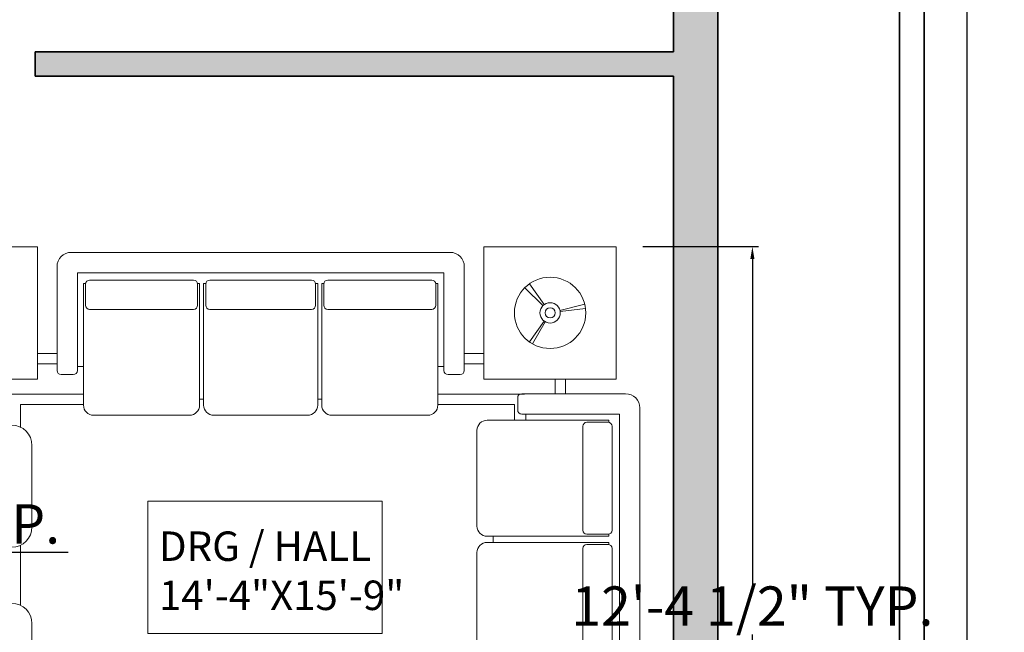
# Model space of a CAD drawing. Units: inches. Extents: x 1070 to 2371, y 645 to 1546.
# Tile 5 of 10: x 1458 to 1658, y 890 to 1014. Entities that reach past the tile are written whole.
import ezdxf

# ---------------------------------------------------------------- set-up
doc = ezdxf.new("R2010")
doc.units = ezdxf.units.IN
for name, color, linetype, lineweight in [('A-ANNO-DIMS', 2, 'Continuous', 18), ('A-AREA-IDEN', 7, 'Continuous', 18), ('A-FURN', 8, 'Continuous', 18), ('A-WALL', 7, 'Continuous', 35), ('C-PROP', 7, 'Continuous', 35)]:
    doc.layers.add(name, color=color, linetype=linetype, lineweight=lineweight)
doc.layers.add('A-WALL-PATT', color=162, linetype='Continuous', lineweight=13, true_color=0x044ac3)
doc.styles.get("Standard").update_dxf_attribs({"font": 'arial.ttf'})
doc.dimstyles.new('ISO-25', dxfattribs={"dimtxt": 8, "dimasz": 2.5, "dimexe": 1.25, "dimexo": 0.625, "dimtad": 1, "dimtih": 1, "dimtoh": 1, "dimdec": 1, "dimlunit": 3, "dimtxsty": 'Standard', "dimcen": 2.5, "dimadec": 0, "dimazin": 0, "dimtfac": 1, "dimtdec": 1, "dimtmove": 0, "dimatfit": 3, "dimfxl": 1, "dimarcsym": 0})

# ---------------------------------------------------------------- blocks, each defined once
blk = doc.blocks.new('A$C71DE5BFE')
for p, q in [((2753, 3552), (893, 3552)), ((823, 3482), (823, 2972)), ((2823, 2972), (2823, 3482)), ((923, 3452), (2723, 3452)), ((923, 2972), (923, 3452)), ((2723, 3452), (2723, 2972)), ((430.7, 3295.7), (503.4, 3397.4)), ((963.5, 3399.9), (953, 3399.9)), ((953, 3399.9), (953, 2802)), ((963, 3292), (963, 3395.7)), ((1493, 3415.7), (983, 3415.7)), ((1523, 3399.9), (1512.6, 3399.9)), ((1513, 3292), (1513, 3395.7)), ((1523, 2802), (1523, 3399.9)), ((1553.5, 3399.9), (1543, 3399.9)), ((1543, 2802), (1543, 3399.9)), ((1553, 3292), (1553, 3395.7)), ((2073, 3415.7), (1573, 3415.7)), ((2103, 3399.9), (2092.6, 3399.9)), ((2093, 3292), (2093, 3395.7)), ((2103, 2802), (2103, 3399.9)), ((2133.5, 3399.9), (2123, 3399.9)), ((2123, 2802), (2123, 3399.9)), ((2133, 3292), (2133, 3395.7)), ((2663, 3415.7), (2153, 3415.7)), ((2693, 3399.9), (2683, 3399.9)), ((2683, 3292), (2683, 3395.7)), ((2693, 2802), (2693, 3399.9)), ((3215.3, 3295.7), (3142.7, 3397.4)), ((437, 3290.4), (525.4, 3378.7)), ((3209, 3290.4), (3120.6, 3378.7)), ((353.2, 3267.1), (231.9, 3297.4)), ((3292.9, 3267.1), (3414.1, 3297.4)), ((352, 3261.2), (228, 3276.7)), ((1493, 3272), (983, 3272)), ((2073, 3272), (1573, 3272)), ((2663, 3272), (2153, 3272)), ((3294, 3261.2), (3418, 3276.7)), ((426.5, 3211.6), (488.5, 3103.1)), ((430.7, 3214.3), (503.4, 3112.6)), ((3215.3, 3214.3), (3142.7, 3112.6)), ((3219.6, 3211.6), (3157.6, 3103.1)), ((726.7, 3055), (823, 3055)), ((2823, 3055), (2919.4, 3055)), ((726.7, 3005), (823, 3005)), ((2823, 3005), (2919.4, 3005)), ((843, 2952), (903, 2952)), ((953, 2992), (923, 2992)), ((2723, 2992), (2693, 2992)), ((2743, 2952), (2803, 2952)), ((394.4, 2753.9), (394.4, 2930)), ((444.4, 2753.9), (444.4, 2930)), ((3269.4, 2930), (3269.4, 2857.9)), ((3319.4, 2930), (3319.4, 2857.9)), ((2693, 2855), (3119.4, 2855)), ((3615.1, 2857.9), (3105.1, 2857.9)), ((1543, 2832), (1523, 2832)), ((2123, 2832), (2103, 2832)), ((2693, 2805), (3069.4, 2805)), ((3069.4, 2805), (3069.4, 2727.9)), ((3085.1, 2837.9), (3085.1, 2777.9)), ((3105.1, 2757.9), (3585.1, 2757.9)), ((3125.1, 2727.9), (3125.1, 2757.9)), ((3585.1, 2757.9), (3585.1, 1527.9)), ((3685.1, 1497.9), (3685.1, 2787.9)), ((350, 2753.9), (510, 2753.9)), ((540, 2723.9), (540, 2703.9)), ((1473, 2752), (1003, 2752)), ((2053, 2752), (1593, 2752)), ((2643, 2752), (2173, 2752)), ((3532.9, 2727.9), (2935.1, 2727.9)), ((3425.1, 2717.9), (3528.7, 2717.9)), ((3532.9, 2717.5), (3532.9, 2727.9)), ((202.1, 2655.3), (206.4, 2659.6)), ((206.4, 2659.6), (210.7, 2661.9)), ((210.7, 2661.9), (213.1, 2666.2)), ((213.1, 2666.2), (217.4, 2668.5)), ((217.4, 2668.5), (219.7, 2672.9)), ((219.7, 2672.9), (224, 2672.9)), ((224, 2672.9), (228.3, 2675.2)), ((228.3, 2675.2), (232.7, 2677.2)), ((232.7, 2677.2), (245.9, 2677.2)), ((245.9, 2677.2), (250.2, 2679.5)), ((250.2, 2679.5), (254.6, 2681.5)), ((254.6, 2681.5), (256.9, 2686.1)), ((256.9, 2686.1), (261.2, 2686.1)), ((261.2, 2686.1), (265.5, 2688.1)), ((265.5, 2688.1), (270.1, 2688.1)), ((270.1, 2688.1), (274.4, 2690.5)), ((272.1, 2657.6), (276.5, 2661.9)), ((274.4, 2690.5), (283.1, 2690.5)), ((276.5, 2661.9), (281.1, 2664.2)), ((281.1, 2664.2), (283.1, 2668.5)), ((283.1, 2690.5), (287.7, 2692.5)), ((283.1, 2668.5), (285.4, 2672.9)), ((285.4, 2672.9), (289.7, 2677.2)), ((287.7, 2692.5), (305, 2692.5)), ((289.7, 2677.2), (292, 2681.5)), ((292, 2659.6), (289.7, 2655.3)), ((292, 2681.5), (296.3, 2686.1)), ((296.3, 2664.2), (292, 2659.6)), ((296.3, 2686.1), (298.6, 2690.5)), ((300.7, 2668.5), (296.3, 2664.2)), ((298.6, 2690.5), (300.7, 2694.8)), ((300.7, 2694.8), (303, 2694.8)), ((305, 2675.2), (300.7, 2668.5)), ((305, 2692.5), (309.6, 2694.8)), ((309.6, 2677.2), (305, 2675.2)), ((309.6, 2694.8), (322.6, 2694.8)), ((311.6, 2681.5), (309.6, 2677.2)), ((315.9, 2683.8), (311.6, 2681.5)), ((320.5, 2686.1), (315.9, 2683.8)), ((318.2, 2697.1), (322.6, 2697.1)), ((322.6, 2690.5), (320.5, 2686.1)), ((322.6, 2694.8), (326.9, 2697.1)), ((322.6, 2697.1), (326.9, 2694.8)), ((326.9, 2694.8), (322.6, 2690.5)), ((326.9, 2697.1), (329.2, 2697.1)), ((326.9, 2694.8), (331.5, 2686.1)), ((331.5, 2686.1), (333.5, 2681.5)), ((333.5, 2681.5), (333.5, 2677.2)), ((333.5, 2677.2), (335.8, 2672.9)), ((335.8, 2659.6), (333.5, 2655.3)), ((335.8, 2672.9), (335.8, 2659.6)), ((350, 2703.9), (600, 2703.9)), ((2885.1, 2207.9), (2885.1, 2677.9)), ((3405.1, 2187.9), (3405.1, 2697.9)), ((3548.7, 2187.9), (3548.7, 2697.9)), ((138.4, 2609.4), (143, 2611.4)), ((143, 2615.7), (147.3, 2618)), ((143, 2611.4), (143, 2615.7)), ((147.3, 2618), (149.4, 2622.4)), ((149.4, 2622.4), (154, 2624.7)), ((154, 2624.7), (158.3, 2626.7)), ((158.3, 2626.7), (162.6, 2631.3)), ((162.6, 2631.3), (166.9, 2635.6)), ((166.9, 2635.6), (171.3, 2637.7)), ((171.3, 2637.7), (175.9, 2640)), ((175.9, 2640), (180.2, 2642.3)), ((180.2, 2642.3), (184.5, 2646.6)), ((184.5, 2646.6), (188.8, 2648.6)), ((188.8, 2648.6), (193.5, 2650.9)), ((193.5, 2650.9), (197.8, 2653.2)), ((197.8, 2653.2), (202.1, 2655.3)), ((239.3, 2611.4), (241.6, 2615.7)), ((239.3, 2607.1), (239.3, 2611.4)), ((241.6, 2615.7), (243.6, 2620.4)), ((243.6, 2620.4), (248.2, 2624.7)), ((248.2, 2624.7), (250.2, 2629)), ((250.2, 2629), (252.5, 2633.3)), ((252.5, 2633.3), (256.9, 2637.7)), ((256.9, 2637.7), (259.2, 2642.3)), ((259.2, 2642.3), (261.2, 2646.6)), ((261.2, 2646.6), (263.5, 2650.9)), ((263.5, 2650.9), (267.8, 2655.3)), ((267.8, 2655.3), (272.1, 2657.6)), ((272.1, 2615.7), (267.8, 2605.1)), ((276.5, 2620.4), (272.1, 2615.7)), ((281.1, 2629), (276.5, 2624.7)), ((276.5, 2624.7), (276.5, 2620.4)), ((283.1, 2633.3), (281.1, 2629)), ((285.4, 2637.7), (283.1, 2633.3)), ((287.7, 2648.6), (285.4, 2644.3)), ((285.4, 2644.3), (285.4, 2637.7)), ((289.7, 2655.3), (287.7, 2648.6)), ((318.2, 2611.4), (315.9, 2607.1)), ((320.5, 2620.4), (318.2, 2615.7)), ((318.2, 2615.7), (318.2, 2611.4)), ((322.6, 2629), (320.5, 2624.7)), ((320.5, 2624.7), (320.5, 2620.4)), ((324.9, 2633.3), (322.6, 2629)), ((329.2, 2637.7), (324.9, 2633.3)), ((331.5, 2646.6), (329.2, 2642.3)), ((329.2, 2642.3), (329.2, 2637.7)), ((333.5, 2650.9), (331.5, 2646.6)), ((333.5, 2655.3), (333.5, 2650.9)), ((99.2, 2561.2), (103.5, 2563.2)), ((103.5, 2563.2), (105.6, 2567.6)), ((105.6, 2567.6), (110.2, 2567.6)), ((110.2, 2572.2), (114.5, 2574.2)), ((110.2, 2567.6), (110.2, 2572.2)), ((114.5, 2574.2), (116.5, 2578.5)), ((116.5, 2578.5), (118.8, 2583.1)), ((118.8, 2583.1), (123.1, 2585.2)), ((123.1, 2589.5), (127.5, 2591.8)), ((123.1, 2585.2), (123.1, 2589.5)), ((127.5, 2591.8), (129.8, 2596.1)), ((129.8, 2596.1), (134.1, 2600.5)), ((134.1, 2600.5), (136.4, 2605.1)), ((136.4, 2605.1), (138.4, 2609.4)), ((226.3, 2561.2), (228.3, 2565.5)), ((228.3, 2565.5), (230.6, 2569.9)), ((230.6, 2574.2), (232.7, 2580.8)), ((230.6, 2569.9), (230.6, 2574.2)), ((232.7, 2589.5), (235, 2594.1)), ((232.7, 2580.8), (232.7, 2589.5)), ((235, 2598.4), (237.3, 2602.8)), ((235, 2594.1), (235, 2598.4)), ((237.3, 2602.8), (239.3, 2607.1)), ((243.6, 2567.6), (241.6, 2561.2)), ((248.2, 2574.2), (243.6, 2567.6)), ((250.2, 2578.5), (248.2, 2574.2)), ((254.6, 2585.2), (250.2, 2578.5)), ((259.2, 2594.1), (254.6, 2585.2)), ((267.8, 2605.1), (259.2, 2594.1)), ((298.6, 2569.9), (294, 2561.2)), ((300.7, 2578.5), (298.6, 2569.9)), ((303, 2585.2), (300.7, 2578.5)), ((311.6, 2598.4), (303, 2589.5)), ((303, 2589.5), (303, 2585.2)), ((315.9, 2607.1), (311.6, 2598.4)), ((700, 2603.9), (700, 2203.9)), ((68.4, 2510.7), (70.7, 2515.1)), ((70.7, 2515.1), (72.7, 2519.4)), ((72.7, 2519.4), (75, 2523.7)), ((75, 2523.7), (79.3, 2528.3)), ((79.3, 2528.3), (83.7, 2530.4)), ((83.7, 2530.4), (86, 2534.7)), ((86, 2534.7), (88.3, 2539.3)), ((88.3, 2539.3), (90.3, 2543.6)), ((90.3, 2543.6), (92.6, 2547.9)), ((92.6, 2547.9), (94.6, 2552.3)), ((94.6, 2552.3), (99.2, 2556.6)), ((99.2, 2556.6), (99.2, 2561.2)), ((210.7, 2515.1), (213.1, 2519.4)), ((210.7, 2510.7), (210.7, 2515.1)), ((213.1, 2519.4), (217.4, 2526)), ((217.4, 2530.4), (219.7, 2534.7)), ((217.4, 2526), (217.4, 2530.4)), ((219.7, 2541.3), (221.7, 2547.9)), ((219.7, 2534.7), (219.7, 2541.3)), ((221.7, 2552.3), (224, 2556.6)), ((221.7, 2547.9), (221.7, 2552.3)), ((224, 2556.6), (226.3, 2561.2)), ((235, 2534.7), (232.7, 2530.4)), ((232.7, 2530.4), (232.7, 2510.7)), ((237.3, 2541.3), (235, 2534.7)), ((239.3, 2552.3), (237.3, 2545.6)), ((237.3, 2545.6), (237.3, 2541.3)), ((241.6, 2561.2), (239.3, 2556.6)), ((239.3, 2556.6), (239.3, 2552.3)), ((289.7, 2528.3), (285.4, 2519.4)), ((285.4, 2519.4), (285.4, 2499.8)), ((292, 2541.3), (289.7, 2534.7)), ((289.7, 2534.7), (289.7, 2528.3)), ((294, 2556.6), (292, 2547.9)), ((292, 2547.9), (292, 2541.3)), ((294, 2561.2), (294, 2556.6)), ((57.4, 2471.2), (59.7, 2475.5)), ((57.4, 2462.6), (57.4, 2471.2)), ((59.7, 2475.5), (61.8, 2480.2)), ((61.8, 2480.2), (64.1, 2484.5)), ((64.1, 2488.8), (66.4, 2493.1)), ((64.1, 2484.5), (64.1, 2488.8)), ((66.4, 2497.5), (68.4, 2502.1)), ((66.4, 2493.1), (66.4, 2497.5)), ((68.4, 2502.1), (68.4, 2510.7)), ((204.4, 2464.6), (206.4, 2469.2)), ((206.4, 2493.1), (208.7, 2497.5)), ((206.4, 2469.2), (206.4, 2493.1)), ((208.7, 2506.4), (210.7, 2510.7)), ((208.7, 2497.5), (208.7, 2506.4)), ((217.4, 2471.2), (215.4, 2466.9)), ((215.4, 2466.9), (215.4, 2436.3)), ((219.7, 2475.5), (217.4, 2471.2)), ((221.7, 2482.2), (219.7, 2475.5)), ((224, 2486.5), (221.7, 2482.2)), ((226.3, 2491.1), (224, 2486.5)), ((228.3, 2497.5), (226.3, 2491.1)), ((230.6, 2504.1), (228.3, 2497.5)), ((232.7, 2510.7), (230.6, 2504.1)), ((285.4, 2499.8), (276.5, 2482.2)), ((276.5, 2482.2), (276.5, 2453.6)), ((55.1, 2423), (57.4, 2427.4)), ((55.1, 2405.4), (55.1, 2423)), ((59.7, 2458.2), (57.4, 2462.6)), ((57.4, 2436.3), (59.7, 2440.6)), ((57.4, 2427.4), (57.4, 2436.3)), ((59.7, 2440.6), (59.7, 2458.2)), ((193.5, 2414.4), (197.8, 2427.4)), ((197.8, 2427.4), (199.8, 2431.7)), ((199.8, 2431.7), (202.1, 2436.3)), ((202.1, 2440.6), (204.4, 2445)), ((202.1, 2436.3), (202.1, 2440.6)), ((204.4, 2445), (204.4, 2464.6)), ((215.4, 2436.3), (206.4, 2418.7)), ((206.4, 2418.7), (206.4, 2392.5)), ((267.8, 2427.4), (259.2, 2410.1)), ((276.5, 2453.6), (267.8, 2445)), ((267.8, 2445), (267.8, 2427.4)), ((53.1, 2401.1), (55.1, 2405.4)), ((53.1, 2392.5), (53.1, 2401.1)), ((55.1, 2388.1), (53.1, 2392.5)), ((55.1, 2361.6), (55.1, 2388.1)), ((184.5, 2377.2), (186.8, 2381.5)), ((184.5, 2363.9), (184.5, 2377.2)), ((186.8, 2392.5), (188.8, 2396.8)), ((186.8, 2381.5), (186.8, 2392.5)), ((188.8, 2401.1), (191.2, 2405.4)), ((188.8, 2396.8), (188.8, 2401.1)), ((191.2, 2405.4), (193.5, 2414.4)), ((197.8, 2372.6), (195.5, 2368.2)), ((206.4, 2392.5), (197.8, 2383.5)), ((197.8, 2383.5), (197.8, 2372.6)), ((250.2, 2370.5), (248.2, 2366.2)), ((259.2, 2392.5), (250.2, 2374.9)), ((250.2, 2374.9), (250.2, 2370.5)), ((259.2, 2410.1), (259.2, 2392.5)), ((57.4, 2357.3), (55.1, 2361.6)), ((57.4, 2352.9), (57.4, 2357.3)), ((59.7, 2348.6), (57.4, 2352.9)), ((59.7, 2344.3), (59.7, 2348.6)), ((61.8, 2340), (59.7, 2344.3)), ((64.1, 2335.3), (61.8, 2340)), ((66.4, 2331), (64.1, 2335.3)), ((66.4, 2326.7), (66.4, 2331)), ((68.4, 2322.4), (66.4, 2326.7)), ((68.4, 2318), (68.4, 2322.4)), ((175.9, 2315.7), (177.9, 2322.4)), ((177.9, 2335.3), (180.2, 2342)), ((177.9, 2322.4), (177.9, 2335.3)), ((180.2, 2350.6), (182.5, 2357.3)), ((180.2, 2342), (180.2, 2350.6)), ((182.5, 2357.3), (184.5, 2363.9)), ((195.5, 2363.9), (193.5, 2359.6)), ((193.5, 2359.6), (193.5, 2274.2)), ((195.5, 2368.2), (195.5, 2363.9)), ((248.2, 2366.2), (248.2, 2307.1)), ((70.7, 2311.4), (68.4, 2318)), ((72.7, 2307.1), (70.7, 2311.4)), ((75, 2302.5), (72.7, 2307.1)), ((77.3, 2298.1), (75, 2302.5)), ((77.3, 2293.8), (77.3, 2298.1)), ((79.3, 2289.5), (77.3, 2293.8)), ((81.6, 2285.1), (79.3, 2289.5)), ((83.7, 2278.5), (81.6, 2285.1)), ((86, 2274.2), (83.7, 2278.5)), ((88.3, 2269.6), (86, 2274.2)), ((175.9, 2311.4), (175.9, 2315.7)), ((177.9, 2307.1), (175.9, 2311.4)), ((177.9, 2298.1), (177.9, 2307.1)), ((180.2, 2293.8), (177.9, 2298.1)), ((180.2, 2254.3), (180.2, 2293.8)), ((193.5, 2274.2), (195.5, 2265.2)), ((248.2, 2307.1), (245.9, 2300.4)), ((245.9, 2300.4), (245.9, 2263.2)), ((90.3, 2265.2), (88.3, 2269.6)), ((94.6, 2263.2), (90.3, 2265.2)), ((96.9, 2258.6), (94.6, 2263.2)), ((101.2, 2256.6), (96.9, 2258.6)), ((103.5, 2252.3), (101.2, 2256.6)), ((107.9, 2250), (103.5, 2252.3)), ((112.2, 2245.6), (107.9, 2250)), ((121.1, 2239), (112.2, 2245.6)), ((134.1, 2226), (121.1, 2239)), ((136.4, 2221.4), (134.1, 2226)), ((182.5, 2250), (180.2, 2254.3)), ((182.5, 2245.6), (182.5, 2250)), ((184.5, 2239), (182.5, 2245.6)), ((184.5, 2212.7), (184.5, 2239)), ((195.5, 2265.2), (195.5, 2252.3)), ((195.5, 2252.3), (197.8, 2247.9)), ((197.8, 2247.9), (197.8, 2243.3)), ((197.8, 2243.3), (199.8, 2232.4)), ((199.8, 2232.4), (199.8, 2215)), ((243.6, 2228), (241.6, 2223.7)), ((245.9, 2237), (243.6, 2232.4)), ((243.6, 2232.4), (243.6, 2228)), ((245.9, 2263.2), (248.2, 2258.6)), ((248.2, 2241.3), (245.9, 2237)), ((248.2, 2258.6), (248.2, 2241.3)), ((140.7, 2219.4), (136.4, 2221.4)), ((143, 2215), (140.7, 2219.4)), ((145, 2210.4), (143, 2215)), ((147.3, 2206.1), (145, 2210.4)), ((149.4, 2201.8), (147.3, 2206.1)), ((151.7, 2197.5), (149.4, 2201.8)), ((154, 2190.8), (151.7, 2197.5)), ((154, 2186.5), (154, 2190.8)), ((156, 2182.2), (154, 2186.5)), ((160.3, 2179.9), (156, 2182.2)), ((162.6, 2175.5), (160.3, 2179.9)), ((186.8, 2208.4), (184.5, 2212.7)), ((186.8, 2204.1), (186.8, 2208.4)), ((188.8, 2199.5), (186.8, 2204.1)), ((188.8, 2190.8), (188.8, 2199.5)), ((191.2, 2186.5), (188.8, 2190.8)), ((191.2, 2179.9), (191.2, 2186.5)), ((193.5, 2175.5), (191.2, 2179.9)), ((199.8, 2215), (202.1, 2208.4)), ((202.1, 2208.4), (202.1, 2186.5)), ((202.1, 2186.5), (204.4, 2182.2)), ((204.4, 2182.2), (204.4, 2173.2)), ((239.3, 2184.2), (237.3, 2179.9)), ((237.3, 2179.9), (237.3, 2175.5)), ((241.6, 2197.5), (239.3, 2193.1)), ((239.3, 2193.1), (239.3, 2184.2)), ((241.6, 2223.7), (241.6, 2197.5)), ((166.9, 2171.2), (162.6, 2175.5)), ((169.2, 2166.6), (166.9, 2171.2)), ((173.6, 2166.6), (169.2, 2166.6)), ((175.9, 2162.3), (173.6, 2166.6)), ((180.2, 2162.3), (175.9, 2162.3)), ((184.5, 2160.2), (180.2, 2162.3)), ((188.8, 2157.9), (184.5, 2160.2)), ((195.5, 2153.6), (188.8, 2157.9)), ((195.5, 2171.2), (193.5, 2175.5)), ((195.5, 2162.3), (195.5, 2171.2)), ((197.8, 2157.9), (195.5, 2162.3)), ((199.8, 2151.3), (195.5, 2153.6)), ((199.8, 2153.6), (197.8, 2157.9)), ((199.8, 2149.3), (199.8, 2153.6)), ((204.4, 2149.3), (199.8, 2151.3)), ((204.4, 2173.2), (206.4, 2168.9)), ((208.7, 2147), (204.4, 2149.3)), ((206.4, 2168.9), (206.4, 2164.6)), ((206.4, 2164.6), (208.7, 2160.2)), ((208.7, 2160.2), (210.7, 2155.9)), ((213.1, 2149.3), (208.7, 2147)), ((210.7, 2155.9), (213.1, 2151.3)), ((213.1, 2151.3), (213.1, 2149.3)), ((226.3, 2149.3), (213.1, 2149.3)), ((228.3, 2153.6), (226.3, 2149.3)), ((232.7, 2157.9), (228.3, 2153.6)), ((235, 2162.3), (232.7, 2157.9)), ((237.3, 2175.5), (235, 2171.2)), ((235, 2171.2), (235, 2162.3)), ((2935.1, 2157.9), (3532.9, 2157.9)), ((2935.1, 2127.9), (3532.9, 2127.9)), ((2965.1, 2137.9), (2965.1, 2157.9)), ((2965.1, 2127.9), (2965.1, 2147.9)), ((3425.1, 2167.9), (3528.7, 2167.9)), ((3532.9, 2157.9), (3532.9, 2168.4)), ((3532.9, 2117.5), (3532.9, 2127.9)), ((350, 2103.9), (600, 2103.9)), ((540, 2103.9), (540, 2083.9)), ((594.4, 1828.9), (594.4, 2103.9)), ((644.4, 1818.6), (644.4, 2114.3)), ((3405.1, 1587.9), (3405.1, 2097.9)), ((3425.1, 2117.9), (3528.7, 2117.9)), ((3548.7, 1587.9), (3548.7, 2097.9)), ((510, 2053.9), (350, 2053.9)), ((394.4, 1878.9), (394.4, 2053.9)), ((444.4, 1878.9), (444.4, 2053.9)), ((2885.1, 1607.9), (2885.1, 2077.9)), ((350, 1878.9), (510, 1878.9)), ((540, 1848.9), (540, 1828.9)), ((210.7, 1786.9), (213.1, 1791.2)), ((213.1, 1791.2), (217.4, 1793.5)), ((217.4, 1793.5), (219.7, 1797.9)), ((219.7, 1797.9), (224, 1797.9)), ((224, 1797.9), (228.3, 1800.2)), ((228.3, 1800.2), (232.7, 1802.2)), ((232.7, 1802.2), (245.9, 1802.2)), ((245.9, 1802.2), (250.2, 1804.5)), ((250.2, 1804.5), (254.6, 1806.5)), ((254.6, 1806.5), (256.9, 1811.1)), ((256.9, 1811.1), (261.2, 1811.1)), ((261.2, 1811.1), (265.5, 1813.1)), ((265.5, 1813.1), (270.1, 1813.1)), ((270.1, 1813.1), (274.4, 1815.5)), ((274.4, 1815.5), (283.1, 1815.5)), ((276.5, 1786.9), (281.1, 1789.2)), ((281.1, 1789.2), (283.1, 1793.5)), ((283.1, 1815.5), (287.7, 1817.5)), ((283.1, 1793.5), (285.4, 1797.9)), ((285.4, 1797.9), (289.7, 1802.2)), ((287.7, 1817.5), (305, 1817.5)), ((289.7, 1802.2), (292, 1806.5)), ((292, 1806.5), (296.3, 1811.1)), ((296.3, 1789.2), (292, 1784.6)), ((296.3, 1811.1), (298.6, 1815.5)), ((300.7, 1793.5), (296.3, 1789.2)), ((298.6, 1815.5), (300.7, 1819.8)), ((300.7, 1819.8), (303, 1819.8)), ((305, 1800.2), (300.7, 1793.5)), ((305, 1817.5), (309.6, 1819.8)), ((309.6, 1802.2), (305, 1800.2)), ((309.6, 1819.8), (322.6, 1819.8)), ((311.6, 1806.5), (309.6, 1802.2)), ((315.9, 1808.8), (311.6, 1806.5)), ((320.5, 1811.1), (315.9, 1808.8)), ((318.2, 1822.1), (322.6, 1822.1)), ((322.6, 1815.5), (320.5, 1811.1)), ((322.6, 1819.8), (326.9, 1822.1)), ((322.6, 1822.1), (326.9, 1819.8)), ((326.9, 1819.8), (322.6, 1815.5)), ((326.9, 1822.1), (329.2, 1822.1)), ((326.9, 1819.8), (331.5, 1811.1)), ((331.5, 1811.1), (333.5, 1806.5)), ((333.5, 1806.5), (333.5, 1802.2)), ((333.5, 1802.2), (335.8, 1797.9)), ((335.8, 1797.9), (335.8, 1784.6)), ((350, 1828.9), (600, 1828.9)), ((143, 1740.7), (147.3, 1743)), ((143, 1736.4), (143, 1740.7)), ((147.3, 1743), (149.4, 1747.4)), ((149.4, 1747.4), (154, 1749.7)), ((154, 1749.7), (158.3, 1751.7)), ((158.3, 1751.7), (162.6, 1756.3)), ((162.6, 1756.3), (166.9, 1760.6)), ((166.9, 1760.6), (171.3, 1762.7)), ((171.3, 1762.7), (175.9, 1765)), ((175.9, 1765), (180.2, 1767.3)), ((180.2, 1767.3), (184.5, 1771.6)), ((184.5, 1771.6), (188.8, 1773.6)), ((188.8, 1773.6), (193.5, 1775.9)), ((193.5, 1775.9), (197.8, 1778.2)), ((197.8, 1778.2), (202.1, 1780.3)), ((202.1, 1780.3), (206.4, 1784.6)), ((206.4, 1784.6), (210.7, 1786.9)), ((239.3, 1736.4), (241.6, 1740.7)), ((241.6, 1740.7), (243.6, 1745.4)), ((243.6, 1745.4), (248.2, 1749.7)), ((248.2, 1749.7), (250.2, 1754)), ((250.2, 1754), (252.5, 1758.3)), ((252.5, 1758.3), (256.9, 1762.7)), ((256.9, 1762.7), (259.2, 1767.3)), ((259.2, 1767.3), (261.2, 1771.6)), ((261.2, 1771.6), (263.5, 1775.9)), ((263.5, 1775.9), (267.8, 1780.3)), ((267.8, 1780.3), (272.1, 1782.6)), ((272.1, 1740.7), (267.8, 1730.1)), ((272.1, 1782.6), (276.5, 1786.9)), ((276.5, 1745.4), (272.1, 1740.7)), ((281.1, 1754), (276.5, 1749.7)), ((276.5, 1749.7), (276.5, 1745.4)), ((283.1, 1758.3), (281.1, 1754)), ((285.4, 1762.7), (283.1, 1758.3)), ((287.7, 1773.6), (285.4, 1769.3)), ((285.4, 1769.3), (285.4, 1762.7)), ((289.7, 1780.3), (287.7, 1773.6)), ((292, 1784.6), (289.7, 1780.3)), ((320.5, 1745.4), (318.2, 1740.7)), ((318.2, 1740.7), (318.2, 1736.4)), ((322.6, 1754), (320.5, 1749.7)), ((320.5, 1749.7), (320.5, 1745.4)), ((324.9, 1758.3), (322.6, 1754)), ((329.2, 1762.7), (324.9, 1758.3)), ((331.5, 1771.6), (329.2, 1767.3)), ((329.2, 1767.3), (329.2, 1762.7)), ((333.5, 1775.9), (331.5, 1771.6)), ((335.8, 1784.6), (333.5, 1780.3)), ((333.5, 1780.3), (333.5, 1775.9)), ((103.5, 1688.2), (105.6, 1692.6)), ((105.6, 1692.6), (110.2, 1692.6)), ((110.2, 1697.2), (114.5, 1699.2)), ((110.2, 1692.6), (110.2, 1697.2)), ((114.5, 1699.2), (116.5, 1703.5)), ((116.5, 1703.5), (118.8, 1708.1)), ((118.8, 1708.1), (123.1, 1710.2)), ((123.1, 1714.5), (127.5, 1716.8)), ((123.1, 1710.2), (123.1, 1714.5)), ((127.5, 1716.8), (129.8, 1721.1)), ((129.8, 1721.1), (134.1, 1725.5)), ((134.1, 1725.5), (136.4, 1730.1)), ((136.4, 1730.1), (138.4, 1734.4)), ((138.4, 1734.4), (143, 1736.4)), ((228.3, 1690.5), (230.6, 1694.9)), ((230.6, 1699.2), (232.7, 1705.8)), ((230.6, 1694.9), (230.6, 1699.2)), ((232.7, 1714.5), (235, 1719.1)), ((232.7, 1705.8), (232.7, 1714.5)), ((235, 1723.4), (237.3, 1727.8)), ((235, 1719.1), (235, 1723.4)), ((237.3, 1727.8), (239.3, 1732.1)), ((239.3, 1732.1), (239.3, 1736.4)), ((243.6, 1692.6), (241.6, 1686.2)), ((248.2, 1699.2), (243.6, 1692.6)), ((250.2, 1703.5), (248.2, 1699.2)), ((254.6, 1710.2), (250.2, 1703.5)), ((259.2, 1719.1), (254.6, 1710.2)), ((267.8, 1730.1), (259.2, 1719.1)), ((298.6, 1694.9), (294, 1686.2)), ((300.7, 1703.5), (298.6, 1694.9)), ((303, 1710.2), (300.7, 1703.5)), ((311.6, 1723.4), (303, 1714.5)), ((303, 1714.5), (303, 1710.2)), ((315.9, 1732.1), (311.6, 1723.4)), ((318.2, 1736.4), (315.9, 1732.1)), ((700, 1728.9), (700, 1328.9)), ((70.7, 1640.1), (72.7, 1644.4)), ((72.7, 1644.4), (75, 1648.7)), ((75, 1648.7), (79.3, 1653.3)), ((79.3, 1653.3), (83.7, 1655.4)), ((83.7, 1655.4), (86, 1659.7)), ((86, 1659.7), (88.3, 1664.3)), ((88.3, 1664.3), (90.3, 1668.6)), ((90.3, 1668.6), (92.6, 1672.9)), ((92.6, 1672.9), (94.6, 1677.3)), ((94.6, 1677.3), (99.2, 1681.6)), ((99.2, 1686.2), (103.5, 1688.2)), ((99.2, 1681.6), (99.2, 1686.2)), ((210.7, 1640.1), (213.1, 1644.4)), ((213.1, 1644.4), (217.4, 1651)), ((217.4, 1655.4), (219.7, 1659.7)), ((217.4, 1651), (217.4, 1655.4)), ((219.7, 1666.3), (221.7, 1672.9)), ((219.7, 1659.7), (219.7, 1666.3)), ((221.7, 1677.3), (224, 1681.6)), ((221.7, 1672.9), (221.7, 1677.3)), ((224, 1681.6), (226.3, 1686.2)), ((226.3, 1686.2), (228.3, 1690.5)), ((235, 1659.7), (232.7, 1655.4)), ((232.7, 1655.4), (232.7, 1635.7)), ((237.3, 1666.3), (235, 1659.7)), ((239.3, 1677.3), (237.3, 1670.6)), ((237.3, 1670.6), (237.3, 1666.3)), ((241.6, 1686.2), (239.3, 1681.6)), ((239.3, 1681.6), (239.3, 1677.3)), ((289.7, 1653.3), (285.4, 1644.4)), ((285.4, 1644.4), (285.4, 1624.8)), ((292, 1666.3), (289.7, 1659.7)), ((289.7, 1659.7), (289.7, 1653.3)), ((294, 1681.6), (292, 1672.9)), ((292, 1672.9), (292, 1666.3)), ((294, 1686.2), (294, 1681.6)), ((57.4, 1596.2), (59.7, 1600.5)), ((57.4, 1587.6), (57.4, 1596.2)), ((59.7, 1600.5), (61.8, 1605.2)), ((61.8, 1605.2), (64.1, 1609.5)), ((64.1, 1613.8), (66.4, 1618.1)), ((64.1, 1609.5), (64.1, 1613.8)), ((66.4, 1622.5), (68.4, 1627.1)), ((66.4, 1618.1), (66.4, 1622.5)), ((68.4, 1635.7), (70.7, 1640.1)), ((68.4, 1627.1), (68.4, 1635.7)), ((206.4, 1618.1), (208.7, 1622.5)), ((206.4, 1594.2), (206.4, 1618.1)), ((208.7, 1631.4), (210.7, 1635.7)), ((208.7, 1622.5), (208.7, 1631.4)), ((210.7, 1635.7), (210.7, 1640.1)), ((217.4, 1596.2), (215.4, 1591.9)), ((219.7, 1600.5), (217.4, 1596.2)), ((221.7, 1607.2), (219.7, 1600.5)), ((224, 1611.5), (221.7, 1607.2)), ((226.3, 1616.1), (224, 1611.5)), ((228.3, 1622.5), (226.3, 1616.1)), ((230.6, 1629.1), (228.3, 1622.5)), ((232.7, 1635.7), (230.6, 1629.1)), ((285.4, 1624.8), (276.5, 1607.2)), ((276.5, 1607.2), (276.5, 1578.6)), ((55.1, 1548), (57.4, 1552.4)), ((55.1, 1530.4), (55.1, 1548)), ((59.7, 1583.2), (57.4, 1587.6)), ((57.4, 1561.3), (59.7, 1565.6)), ((57.4, 1552.4), (57.4, 1561.3)), ((59.7, 1565.6), (59.7, 1583.2)), ((193.5, 1539.4), (197.8, 1552.4)), ((197.8, 1552.4), (199.8, 1556.7)), ((199.8, 1556.7), (202.1, 1561.3)), ((202.1, 1565.6), (204.4, 1570)), ((202.1, 1561.3), (202.1, 1565.6)), ((204.4, 1589.6), (206.4, 1594.2)), ((204.4, 1570), (204.4, 1589.6)), ((215.4, 1561.3), (206.4, 1543.7)), ((215.4, 1591.9), (215.4, 1561.3)), ((267.8, 1552.4), (259.2, 1535.1)), ((276.5, 1578.6), (267.8, 1570)), ((267.8, 1570), (267.8, 1552.4)), ((2935.1, 1557.9), (3532.9, 1557.9)), ((3125.1, 1527.9), (3125.1, 1557.9)), ((3425.1, 1567.9), (3528.7, 1567.9)), ((3532.9, 1557.9), (3532.9, 1567.9)), ((53.1, 1526.1), (55.1, 1530.4)), ((53.1, 1517.5), (53.1, 1526.1)), ((55.1, 1513.1), (53.1, 1517.5)), ((55.1, 1486.6), (55.1, 1513.1)), ((184.5, 1502.2), (186.8, 1506.5)), ((184.5, 1488.9), (184.5, 1502.2)), ((186.8, 1517.5), (188.8, 1521.8)), ((186.8, 1506.5), (186.8, 1517.5)), ((188.8, 1526.1), (191.2, 1530.4)), ((188.8, 1521.8), (188.8, 1526.1)), ((191.2, 1530.4), (193.5, 1539.4)), ((206.4, 1517.5), (197.8, 1508.5)), ((197.8, 1508.5), (197.8, 1497.6)), ((206.4, 1543.7), (206.4, 1517.5)), ((259.2, 1517.5), (250.2, 1499.9)), ((250.2, 1499.9), (250.2, 1495.5)), ((259.2, 1535.1), (259.2, 1517.5)), ((3085.1, 1507.9), (3085.1, 1447.9)), ((3585.1, 1527.9), (3105.1, 1527.9)), ((57.4, 1482.3), (55.1, 1486.6)), ((57.4, 1477.9), (57.4, 1482.3)), ((59.7, 1473.6), (57.4, 1477.9)), ((59.7, 1469.3), (59.7, 1473.6)), ((61.8, 1465), (59.7, 1469.3)), ((64.1, 1460.3), (61.8, 1465)), ((66.4, 1456), (64.1, 1460.3)), ((66.4, 1451.7), (66.4, 1456)), ((68.4, 1447.4), (66.4, 1451.7)), ((177.9, 1460.3), (180.2, 1467)), ((177.9, 1447.4), (177.9, 1460.3)), ((180.2, 1475.6), (182.5, 1482.3)), ((180.2, 1467), (180.2, 1475.6)), ((182.5, 1482.3), (184.5, 1488.9)), ((195.5, 1488.9), (193.5, 1484.6)), ((193.5, 1484.6), (193.5, 1399.2)), ((197.8, 1497.6), (195.5, 1493.2)), ((195.5, 1493.2), (195.5, 1488.9)), ((250.2, 1495.5), (248.2, 1491.2)), ((248.2, 1491.2), (248.2, 1432.1)), ((68.4, 1443), (68.4, 1447.4)), ((70.7, 1436.4), (68.4, 1443)), ((72.7, 1432.1), (70.7, 1436.4)), ((75, 1427.5), (72.7, 1432.1)), ((77.3, 1423.1), (75, 1427.5)), ((77.3, 1418.8), (77.3, 1423.1)), ((79.3, 1414.5), (77.3, 1418.8)), ((81.6, 1410.1), (79.3, 1414.5)), ((83.7, 1403.5), (81.6, 1410.1)), ((86, 1399.2), (83.7, 1403.5)), ((175.9, 1440.7), (177.9, 1447.4)), ((175.9, 1436.4), (175.9, 1440.7)), ((177.9, 1432.1), (175.9, 1436.4)), ((177.9, 1423.1), (177.9, 1432.1)), ((180.2, 1418.8), (177.9, 1423.1)), ((180.2, 1379.3), (180.2, 1418.8)), ((248.2, 1432.1), (245.9, 1425.4)), ((245.9, 1425.4), (245.9, 1388.2)), ((3105.1, 1427.9), (3615.1, 1427.9)), ((88.3, 1394.6), (86, 1399.2)), ((90.3, 1390.2), (88.3, 1394.6)), ((94.6, 1388.2), (90.3, 1390.2)), ((96.9, 1383.6), (94.6, 1388.2)), ((101.2, 1381.6), (96.9, 1383.6)), ((103.5, 1377.3), (101.2, 1381.6)), ((107.9, 1375), (103.5, 1377.3)), ((112.2, 1370.6), (107.9, 1375)), ((121.1, 1364), (112.2, 1370.6)), ((134.1, 1351), (121.1, 1364)), ((182.5, 1375), (180.2, 1379.3)), ((182.5, 1370.6), (182.5, 1375)), ((184.5, 1364), (182.5, 1370.6)), ((184.5, 1337.7), (184.5, 1364)), ((193.5, 1399.2), (195.5, 1390.2)), ((195.5, 1390.2), (195.5, 1377.3)), ((195.5, 1377.3), (197.8, 1372.9)), ((197.8, 1372.9), (197.8, 1368.3)), ((197.8, 1368.3), (199.8, 1357.4)), ((199.8, 1357.4), (199.8, 1340)), ((245.9, 1362), (243.6, 1357.4)), ((243.6, 1357.4), (243.6, 1353)), ((245.9, 1388.2), (248.2, 1383.6)), ((248.2, 1366.3), (245.9, 1362)), ((248.2, 1383.6), (248.2, 1366.3)), ((136.4, 1346.4), (134.1, 1351)), ((140.7, 1344.4), (136.4, 1346.4)), ((143, 1340), (140.7, 1344.4)), ((145, 1335.4), (143, 1340)), ((147.3, 1331.1), (145, 1335.4)), ((149.4, 1326.8), (147.3, 1331.1)), ((151.7, 1322.5), (149.4, 1326.8)), ((154, 1315.8), (151.7, 1322.5)), ((154, 1311.5), (154, 1315.8)), ((156, 1307.2), (154, 1311.5)), ((160.3, 1304.9), (156, 1307.2)), ((186.8, 1333.4), (184.5, 1337.7)), ((186.8, 1329.1), (186.8, 1333.4)), ((188.8, 1324.5), (186.8, 1329.1)), ((188.8, 1315.8), (188.8, 1324.5)), ((191.2, 1311.5), (188.8, 1315.8)), ((191.2, 1304.9), (191.2, 1311.5)), ((199.8, 1340), (202.1, 1333.4)), ((202.1, 1333.4), (202.1, 1311.5)), ((202.1, 1311.5), (204.4, 1307.2)), ((204.4, 1307.2), (204.4, 1298.2)), ((239.3, 1309.2), (237.3, 1304.9)), ((241.6, 1322.5), (239.3, 1318.1)), ((239.3, 1318.1), (239.3, 1309.2)), ((243.6, 1353), (241.6, 1348.7)), ((241.6, 1348.7), (241.6, 1322.5)), ((162.6, 1300.5), (160.3, 1304.9)), ((166.9, 1296.2), (162.6, 1300.5)), ((169.2, 1291.6), (166.9, 1296.2)), ((173.6, 1291.6), (169.2, 1291.6)), ((175.9, 1287.3), (173.6, 1291.6)), ((180.2, 1287.3), (175.9, 1287.3)), ((184.5, 1285.2), (180.2, 1287.3)), ((188.8, 1282.9), (184.5, 1285.2)), ((195.5, 1278.6), (188.8, 1282.9)), ((193.5, 1300.5), (191.2, 1304.9)), ((195.5, 1296.2), (193.5, 1300.5)), ((195.5, 1287.3), (195.5, 1296.2)), ((197.8, 1282.9), (195.5, 1287.3)), ((199.8, 1276.3), (195.5, 1278.6)), ((199.8, 1278.6), (197.8, 1282.9)), ((199.8, 1274.3), (199.8, 1278.6)), ((204.4, 1274.3), (199.8, 1276.3)), ((204.4, 1298.2), (206.4, 1293.9)), ((208.7, 1272), (204.4, 1274.3)), ((206.4, 1293.9), (206.4, 1289.6)), ((206.4, 1289.6), (208.7, 1285.2)), ((208.7, 1285.2), (210.7, 1280.9)), ((213.1, 1274.3), (208.7, 1272)), ((210.7, 1280.9), (213.1, 1276.3)), ((213.1, 1276.3), (213.1, 1274.3)), ((226.3, 1274.3), (213.1, 1274.3)), ((228.3, 1278.6), (226.3, 1274.3)), ((232.7, 1282.9), (228.3, 1278.6)), ((235, 1287.3), (232.7, 1282.9)), ((237.3, 1300.5), (235, 1296.2)), ((235, 1296.2), (235, 1287.3)), ((237.3, 1304.9), (237.3, 1300.5)), ((350, 1228.9), (600, 1228.9)), ((540, 1228.9), (540, 1208.9)), ((510, 1178.9), (350, 1178.9)), ((1322.3, 1189.3), (1792.3, 1189.3)), ((1922.3, 1189.3), (2392.3, 1189.3)), ((1272.3, 1139.3), (1272.3, 541.4)), ((1842.3, 1139.3), (1842.3, 541.4)), ((1872.3, 1139.3), (1872.3, 541.4)), ((2442.3, 541.4), (2442.3, 1139.3)), ((1842.3, 1109.3), (1862.3, 1109.3)), ((1852.3, 1109.3), (1872.3, 1109.3)), ((1142.3, 969.3), (1142.3, 459.3)), ((1222.3, 989.3), (1162.3, 989.3)), ((1242.3, 489.3), (1242.3, 969.3)), ((2472.3, 969.3), (2472.3, 489.3)), ((2552.3, 989.3), (2492.3, 989.3)), ((2572.3, 459.3), (2572.3, 969.3)), ((1242.3, 949.3), (1272.3, 949.3)), ((2442.3, 949.3), (2472.3, 949.3)), ((1282.3, 649.3), (1282.3, 545.6)), ((1302.3, 669.3), (1812.3, 669.3)), ((1832.3, 649.3), (1832.3, 545.6)), ((1882.3, 649.3), (1882.3, 545.6)), ((1902.3, 669.3), (2412.3, 669.3)), ((2432.3, 649.3), (2432.3, 545.6)), ((1272.3, 541.4), (1282.3, 541.4)), ((1831.9, 541.4), (1842.3, 541.4)), ((1872.3, 541.4), (1882.7, 541.4)), ((2431.9, 541.4), (2442.3, 541.4)), ((2472.3, 489.3), (1242.3, 489.3)), ((1302.3, 525.6), (1812.3, 525.6)), ((1902.3, 525.6), (2412.3, 525.6)), ((1212.3, 389.3), (2502.3, 389.3))]:
    blk.add_line(p, q)
for points in [[(726.7, 2930), (76.7, 2930), (76.7, 3580), (726.7, 3580)], [(2919.4, 2930), (3569.4, 2930), (3569.4, 3580), (2919.4, 3580)], [(2419.4, 1680), (2419.4, 2330), (1269.4, 2330), (1269.4, 1680)], [(2464.4, 0), (2464.4, 345), (1264.4, 345), (1264.4, 0)]]:
    blk.add_lwpolyline(points, close=True)
for points in [[(594.4, 2703.9), (594.4, 2855), (953, 2855)], [(644.4, 2693.6), (644.4, 2805), (953, 2805)], [(3069.4, 1557.9), (3069.4, 830), (2572.3, 830)], [(3269.4, 1427.9), (3269.4, 630), (2572.3, 630)], [(3319.4, 1427.9), (3319.4, 580), (2572.3, 580)], [(3119.4, 1427.9), (3119.4, 780), (2572.3, 780)], [(1142.3, 780), (594.4, 780), (594.4, 1228.9)], [(1142.3, 830), (644.4, 830), (644.4, 1239.3)], [(1142.3, 580), (394.4, 580), (394.4, 1178.9)], [(1142.3, 630), (444.4, 630), (444.4, 1178.9)]]:
    blk.add_lwpolyline(points)
for centre, radius in [((401.7, 3255), 175), ((3244.4, 3255), 175), ((401.7, 3255), 50), ((3244.4, 3255), 50), ((401.7, 3255), 25), ((3244.4, 3255), 25)]:
    blk.add_circle(centre, radius)
for centre, radius, start, end in [((893, 3482), 70, 90, 180), ((2753, 3482), 70, 0, 90), ((983, 3395.7), 20, 90, 180), ((1493, 3395.7), 20, 0, 90), ((1573, 3395.7), 20, 90, 180), ((2073, 3395.7), 20, 0, 90), ((2153, 3395.7), 20, 90, 180), ((2663, 3395.7), 20, 0, 90), ((983, 3292), 20, 180, 270), ((1493, 3292), 20, 270, 0), ((1573, 3292), 20, 180, 270), ((2073, 3292), 20, 270, 0), ((2153, 3292), 20, 180, 270), ((2663, 3292), 20, 270, 0), ((843, 2972), 20, 180, 270), ((903, 2972), 20, 270, 0), ((2743, 2972), 20, 180, 270), ((2803, 2972), 20, 270, 0), ((3105.1, 2837.9), 20, 90, 180), ((3615.1, 2787.9), 70, 0, 90), ((1003, 2802), 50, 180, 270), ((1473, 2802), 50, 270, 0), ((1593, 2802), 50, 180, 270), ((2053, 2802), 50, 270, 0), ((2173, 2802), 50, 180, 270), ((2643, 2802), 50, 270, 0), ((3105.1, 2777.9), 20, 180, 270), ((350, 2403.9), 350, 90, 270), ((510, 2723.9), 30, 0, 90), ((2935.1, 2677.9), 50, 90, 180), ((3425.1, 2697.9), 20, 90, 180), ((3528.7, 2697.9), 20, 0, 90), ((350, 2403.9), 300, 90, 270), ((600, 2603.9), 100, 0, 90), ((600, 2203.9), 100, 270, 0), ((2935.1, 2207.9), 50, 180, 270), ((3425.1, 2187.9), 20, 180, 270), ((3528.7, 2187.9), 20, 270, 0), ((2935.1, 2077.9), 50, 90, 180), ((510, 2083.9), 30, 270, 0), ((3425.1, 2097.9), 20, 90, 180), ((3528.7, 2097.9), 20, 0, 90), ((350, 1528.9), 350, 90, 270), ((510, 1848.9), 30, 0, 90), ((350, 1528.9), 300, 90, 270), ((600, 1728.9), 100, 0, 90), ((2935.1, 1607.9), 50, 180, 270), ((3425.1, 1587.9), 20, 180, 270), ((3528.7, 1587.9), 20, 270, 0), ((3105.1, 1507.9), 20, 90, 180), ((3615.1, 1497.9), 70, 270, 0), ((3105.1, 1447.9), 20, 180, 270), ((600, 1328.9), 100, 270, 0), ((510, 1208.9), 30, 270, 0), ((1322.3, 1139.3), 50, 90, 180), ((1792.3, 1139.3), 50, 0, 90), ((1922.3, 1139.3), 50, 90, 180), ((2392.3, 1139.3), 50, 0, 90), ((1162.3, 969.3), 20, 90, 180), ((1222.3, 969.3), 20, 0, 90), ((2492.3, 969.3), 20, 90, 180), ((2552.3, 969.3), 20, 0, 90), ((1302.3, 649.3), 20, 90, 180), ((1812.3, 649.3), 20, 0, 90), ((1902.3, 649.3), 20, 90, 180), ((2412.3, 649.3), 20, 0, 90), ((1302.3, 545.6), 20, 180, 270), ((1812.3, 545.6), 20, 270, 0), ((1902.3, 545.6), 20, 180, 270), ((2412.3, 545.6), 20, 270, 0), ((1212.3, 459.3), 70, 180, 270), ((2502.3, 459.3), 70, 270, 0)]:
    blk.add_arc(centre, radius, start, end)
blk = doc.blocks.new('*D12')
at = {"layer": 'A-ANNO-DIMS', "color": 0, "lineweight": -2, "transparency": 16777216}
for p, q in [((1642.74, 1408.77), (1652.12, 1408.77)), ((1650.87, 1406.27), (1650.87, 1053.48)), ((1650.87, 691.27), (1650.87, 1044.06)), ((1642.74, 688.77), (1652.12, 688.77))]:
    blk.add_line(p, q, dxfattribs=at)
at = {"layer": 'A-ANNO-DIMS', "color": 0, "transparency": 16777216}
for points in [[(1650.46, 1406.27), (1651.29, 1406.27), (1650.87, 1408.77)], [(1650.46, 691.27), (1651.29, 691.27), (1650.87, 688.77)]]:
    blk.add_solid(points, dxfattribs=at)
at = {"layer": 'Defpoints', "color": 0, "transparency": 16777216}
for p in [(1642.11, 1408.77), (1642.11, 688.77), (1650.87, 688.77)]:
    blk.add_point(p, dxfattribs=at)
at = {"layer": 'A-ANNO-DIMS', "color": 0, "transparency": 16777216, "insert": (1650.87, 1048.77), "char_height": 8, "attachment_point": 5}
blk.add_mtext("60'", dxfattribs=at)
blk = doc.blocks.new('*D36')
at = {"layer": 'A-ANNO-DIMS', "color": 0, "lineweight": -2, "transparency": 16777216}
for p, q in [((1584.86, 968.08), (1608.4, 968.08)), ((1607.15, 965.58), (1607.15, 898.62)), ((1607.15, 822.13), (1607.15, 889.1)), ((1584.86, 819.63), (1608.4, 819.63))]:
    blk.add_line(p, q, dxfattribs=at)
at = {"layer": 'A-ANNO-DIMS', "color": 0, "transparency": 16777216}
for points in [[(1606.73, 965.58), (1607.57, 965.58), (1607.15, 968.08)], [(1606.73, 822.13), (1607.57, 822.13), (1607.15, 819.63)]]:
    blk.add_solid(points, dxfattribs=at)
at = {"layer": 'Defpoints', "color": 0, "transparency": 16777216}
for p in [(1584.23, 968.08), (1607.15, 968.08), (1584.23, 819.63)]:
    blk.add_point(p, dxfattribs=at)
at = {"layer": 'A-ANNO-DIMS', "color": 0, "transparency": 16777216, "insert": (1607.15, 893.86), "char_height": 8, "attachment_point": 5}
blk.add_mtext('12\'-4 1/2" TYP.', dxfattribs=at)
blk = doc.blocks.new('*D39')
at = {"layer": 'A-ANNO-DIMS', "color": 0, "lineweight": -2, "transparency": 16777216}
for p, q in [((1359.11, 910.65), (1359.11, 904.62)), ((1395.11, 910.65), (1395.11, 904.62)), ((1361.61, 905.87), (1392.61, 905.87)), ((1395.11, 905.87), (1467.82, 905.87))]:
    blk.add_line(p, q, dxfattribs=at)
at = {"layer": 'A-ANNO-DIMS', "color": 0, "transparency": 16777216}
for points in [[(1361.61, 906.29), (1361.61, 905.46), (1359.11, 905.87)], [(1392.61, 906.29), (1392.61, 905.46), (1395.11, 905.87)]]:
    blk.add_solid(points, dxfattribs=at)
at = {"layer": 'Defpoints', "color": 0, "transparency": 16777216}
for p in [(1359.11, 911.27), (1395.11, 911.27), (1395.11, 905.87)]:
    blk.add_point(p, dxfattribs=at)
at = {"layer": 'A-ANNO-DIMS', "color": 0, "transparency": 16777216, "insert": (1432.72, 910.58), "char_height": 8, "attachment_point": 5}
blk.add_mtext('W3 3\'-0" TYP.', dxfattribs=at)

msp = doc.modelspace()

# ---------------------------------------------------------------- hatches: boundary and pattern name
at = {"layer": 'A-WALL-PATT'}
h = msp.add_hatch(color=256, dxfattribs=at)
h.dxf.hatch_style = 1
h.paths.add_polyline_path([(1245.11, 1097.27), (1236.11, 1097.27), (1236.11, 1043.77), (1245.11, 1043.77)])
h.paths.add_polyline_path([(1245.11, 1198.77), (1207.11, 1198.77), (1207.11, 1333.77), (1245.61, 1333.77), (1245.61, 1342.77), (1198.11, 1342.77), (1198.11, 1189.77), (1236.11, 1189.77), (1236.11, 1145.27), (1245.11, 1145.27)])
h.paths.add_polyline_path([(1344.11, 1342.77), (1305.61, 1342.77), (1305.61, 1333.77), (1344.11, 1333.77)], flags=0)
h.paths.add_polyline_path([(1413.11, 1342.77), (1380.11, 1342.77), (1380.11, 1234.77), (1389.11, 1234.77), (1389.11, 1333.77), (1413.11, 1333.77)], flags=17)
h.paths.add_polyline_path([(1470.11, 1342.77), (1437.11, 1342.77), (1437.11, 1333.77), (1461.11, 1333.77), (1461.11, 1262.77), (1419.11, 1262.77), (1419.11, 1257.77), (1461.11, 1257.77), (1461.11, 1198.77), (1380.11, 1198.77), (1281.11, 1198.77), (1281.11, 1189.77), (1470.11, 1189.77)])
h.paths.add_polyline_path([(1524.61, 1300.77), (1506.11, 1300.77), (1506.11, 1291.77), (1524.61, 1291.77)], flags=17)
h.paths.add_polyline_path([(1600.11, 1300.77), (1572.61, 1300.77), (1572.61, 1291.77), (1591.11, 1291.77), (1591.11, 1152.77), (1461.11, 1152.77), (1461.11, 1143.77), (1567.11, 1143.77), (1567.11, 1131.77), (1576.11, 1131.77), (1576.11, 1143.77), (1600.11, 1143.77)])
h.paths.add_polyline_path([(1600.11, 1071.77), (1576.11, 1071.77), (1576.11, 1083.77), (1567.11, 1083.77), (1567.11, 1071.77), (1461.11, 1071.77), (1461.11, 1043.77), (1466.11, 1043.77), (1466.11, 1066.77), (1508.11, 1066.77), (1508.11, 1037.77), (1513.11, 1037.77), (1513.11, 1062.77), (1591.11, 1062.77), (1591.11, 1047.27), (1600.11, 1047.27)])
h.paths.add_polyline_path([(1600.11, 1023.27), (1591.11, 1023.27), (1591.11, 1007.77), (1461.11, 1007.77), (1461.11, 1002.77), (1591.11, 1002.77), (1591.11, 813.77), (1550.11, 813.77), (1550.11, 804.77), (1600.11, 804.77)])
h.paths.add_polyline_path([(1502.11, 813.77), (1461.11, 813.77), (1461.11, 804.77), (1502.11, 804.77)], flags=0)
h.paths.add_polyline_path([(1419.11, 1007.77), (1395.11, 1007.77), (1395.11, 998.77), (1410.11, 998.77), (1410.11, 916.77), (1395.11, 916.77), (1395.11, 907.77), (1410.11, 907.77), (1410.11, 804.77), (1419.11, 804.77)])

# ---------------------------------------------------------------- linework, layer by layer
at = {"layer": 'A-WALL'}
for p, q in [((1600.11, 1071.77), (1600.11, 804.77)), ((1591.11, 1062.77), (1591.11, 1007.77)), ((1461.11, 1007.77), (1591.11, 1007.77)), ((1461.11, 1002.77), (1461.11, 1007.77)), ((1461.11, 1002.77), (1591.11, 1002.77)), ((1591.11, 1002.77), (1591.11, 813.77))]:
    msp.add_line(p, q, dxfattribs=at)
at = {"layer": 'C-PROP'}
for p, q in [((1642.11, 1408.77), (1642.11, 688.77)), ((1637.11, 1403.77), (1637.11, 693.77))]:
    msp.add_line(p, q, dxfattribs=at)

# ---------------------------------------------------------------- block references
at = {"layer": 'A-FURN', "xscale": 0.0414658939784557, "yscale": 0.0414658939784557, "zscale": 0.0414658939784557}
msp.add_blockref('A$C71DE5BFE', (1431.43, 819.63), dxfattribs=at)

# ---------------------------------------------------------------- texts
at = {"layer": 'A-AREA-IDEN', "insert": (1486.32, 910.09), "char_height": 6, "attachment_point": 1}
msp.add_mtext_dynamic_manual_height_columns('DRG / HALL\\P14\'-4"X15\'-9"', width=62.3796, gutter_width=12.5, heights=[0], dxfattribs=at)

# ---------------------------------------------------------------- dimensions: what is measured, and where the dimension line sits
at = {"layer": 'A-ANNO-DIMS'}
dim = msp.add_linear_dim(base=(1650.87, 688.77), p1=(1642.11, 1408.77), p2=(1642.11, 688.77), angle=90, dimstyle='ISO-25', override={"dimclrd": 0, "dimclre": 0, "dimclrt": 0}, dxfattribs=at)
dim.commit()
dim.dimension.update_dxf_attribs({"geometry": '*D12', "text_midpoint": (1650.87, 1048.77)})
dim = msp.add_linear_dim(base=(1607.1511, 968.0817), p1=(1584.2304, 819.6338), p2=(1584.2304, 968.0817), angle=90, text='<> TYP.', dimstyle='ISO-25', override={"dimdec": 1, "dimlfac": 1, "dimrnd": 0, "dimzin": 1, "dimdsep": 46, "dimlunit": 4, "dimfrac": 2}, dxfattribs=at)
dim.commit()
dim.dimension.update_dxf_attribs({"geometry": '*D36', "text_midpoint": (1607.1511, 893.8578)})
dim = msp.add_linear_dim(base=(1395.11, 905.87), p1=(1359.11, 911.27), p2=(1395.11, 911.27), text='W3 <> TYP.', dimstyle='ISO-25', override={"dimdec": 1, "dimlfac": 1, "dimrnd": 0, "dimzin": 1, "dimdsep": 46, "dimlunit": 4, "dimfrac": 2}, dxfattribs=at)
dim.commit()
dim.dimension.update_dxf_attribs({"geometry": '*D39', "text_midpoint": (1432.72, 910.58)})

doc.saveas('drawing.dxf')
